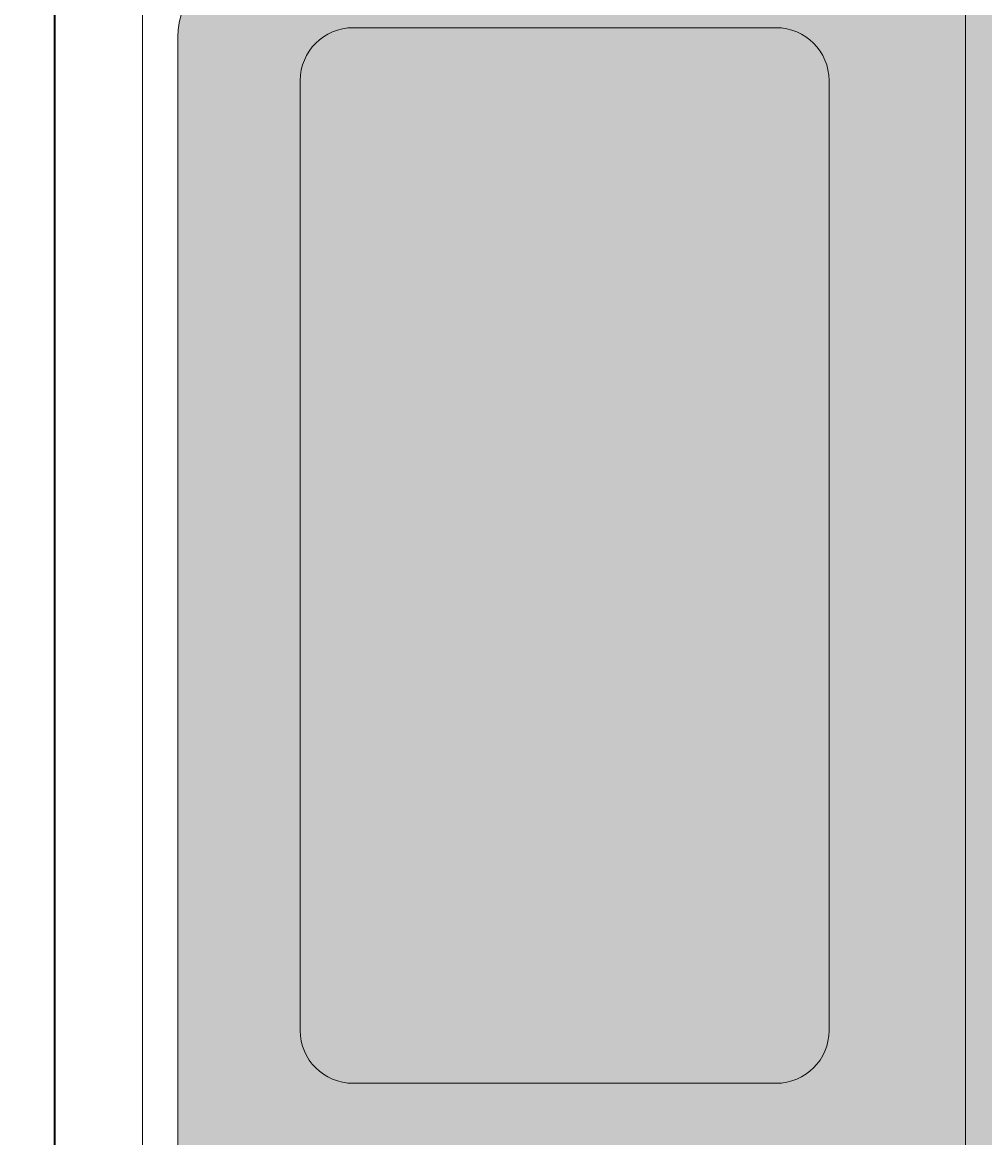
# Model space of a CAD drawing. Units: millimetres. Extents: x 27017497 to 27018854, y 7058029 to 7059154.
# Tile 83 of 91: x 27018319 to 27018341, y 7058530 to 7058555. Entities that reach past the tile are written whole.
import ezdxf

# ---------------------------------------------------------------- set-up
doc = ezdxf.new("R2010")
doc.units = ezdxf.units.MM
for name, color, linetype, lineweight in [('A-ANNO-DIMS', 2, 'Continuous', 18), ('A-FURN', 8, 'Continuous', 18), ('A-WALL', 7, 'Continuous', 35)]:
    doc.layers.add(name, color=color, linetype=linetype, lineweight=lineweight)
doc.layers.add('A-FURN-PATT', color=177, linetype='Continuous', lineweight=13, true_color=0x293189)
doc.styles.get("Standard").update_dxf_attribs({"font": 'arial.ttf'})
doc.dimstyles.get("Standard").update_dxf_attribs({"dimtxt": 0.18, "dimasz": 0.18, "dimexe": 0.18, "dimexo": 0.0625, "dimgap": 0.09, "dimtad": 0, "dimtih": 1, "dimtoh": 1, "dimdec": 4, "dimzin": 0, "dimdsep": 46, "dimtxsty": 'Standard', "dimcen": 0.09, "dimadec": 0, "dimazin": 0, "dimtfac": 1, "dimtdec": 4, "dimtofl": 0, "dimtmove": 0, "dimatfit": 3, "dimfxl": 1, "dimtolj": 1, "dimtzin": 0, "dimarcsym": 0})

# ---------------------------------------------------------------- blocks, each defined once
blk = doc.blocks.new('CAMMAT')
for p, q in [((1.27313, 0), (-1.27313, 0)), ((1.27313, -0.05), (-1.27313, -0.05)), ((0.61, -0.07), (-0.61, -0.07)), ((-0.04645, -0.1395), (-0.58524, -0.1395)), ((-0.61524, -0.1695), (-0.61524, -0.4095)), ((-0.01645, -0.1695), (-0.01645, -0.4095)), ((-0.04645, -0.4395), (-0.58524, -0.4395)), ((-0.6904, -0.51693), (0.68256, -0.51693))]:
    blk.add_line(p, q)
for centre, radius, start, end in [((-0.61, -0.11), 0.04, 90, 180), ((-0.58524, -0.1695), 0.03, 90, 180), ((-0.04645, -0.1695), 0.03, 360, 90), ((-0.58524, -0.4095), 0.03, 180, 270), ((-0.04645, -0.4095), 0.03, 270, 360)]:
    blk.add_arc(centre, radius, start, end)
blk = doc.blocks.new('*D48')
at = {"layer": 'A-ANNO-DIMS', "color": 0, "lineweight": -2, "transparency": 16777216}
for p, q in [((27018463.498, 7058622.912), (27017497.536, 7058622.912)), ((27017497.716, 7058622.732), (27017497.716, 7058357.753)), ((27017497.716, 7058092.41), (27017497.716, 7058357.389)), ((27018555.129, 7058092.23), (27017497.536, 7058092.23))]:
    blk.add_line(p, q, dxfattribs=at)
at = {"layer": 'A-ANNO-DIMS', "color": 0, "transparency": 16777216}
for points in [[(27017497.686, 7058622.732), (27017497.746, 7058622.732), (27017497.716, 7058622.912)], [(27017497.686, 7058092.41), (27017497.746, 7058092.41), (27017497.716, 7058092.23)]]:
    blk.add_solid(points, dxfattribs=at)
at = {"layer": 'Defpoints', "color": 0, "transparency": 16777216}
for p in [(27018463.561, 7058622.912), (27017497.716, 7058092.23), (27018555.192, 7058092.23)]:
    blk.add_point(p, dxfattribs=at)
at = {"layer": 'A-ANNO-DIMS', "color": 0, "transparency": 16777216, "insert": (27017497.716, 7058357.571), "char_height": 0.18, "attachment_point": 5}
blk.add_mtext('\\A1;530.7', dxfattribs=at)
blk = doc.blocks.new('*D50')
at = {"layer": 'A-ANNO-DIMS', "color": 0, "lineweight": -2, "transparency": 16777216}
for p, q in [((27018223.668, 7058580.912), (27018854.236, 7058580.912)), ((27018854.056, 7058580.732), (27018854.056, 7058511.344)), ((27018854.056, 7058441.592), (27018854.056, 7058510.98)), ((27018223.668, 7058441.412), (27018854.236, 7058441.412))]:
    blk.add_line(p, q, dxfattribs=at)
at = {"layer": 'A-ANNO-DIMS', "color": 0, "transparency": 16777216}
for points in [[(27018854.026, 7058580.732), (27018854.086, 7058580.732), (27018854.056, 7058580.912)], [(27018854.026, 7058441.592), (27018854.086, 7058441.592), (27018854.056, 7058441.412)]]:
    blk.add_solid(points, dxfattribs=at)
at = {"layer": 'Defpoints', "color": 0, "transparency": 16777216}
for p in [(27018223.606, 7058580.912), (27018223.606, 7058441.412), (27018854.056, 7058441.412)]:
    blk.add_point(p, dxfattribs=at)
at = {"layer": 'A-ANNO-DIMS', "color": 0, "transparency": 16777216, "insert": (27018854.056, 7058511.162), "char_height": 0.18, "attachment_point": 5}
blk.add_mtext('\\A1;139.5', dxfattribs=at)

msp = doc.modelspace()

# ---------------------------------------------------------------- hatches: boundary and pattern name
at = {"layer": 'A-FURN-PATT'}
h = msp.add_hatch(color=256, dxfattribs=at)
h.dxf.hatch_style = 1
h.paths.add_polyline_path([(27018398.067, 7058554.497, 0.414214), (27018396.474, 7058556.09), (27018352.018, 7058556.09), (27018352.202, 7058552.834), (27018352.581, 7058547.929), (27018353.082, 7058544.346), (27018353.818, 7058541.828), (27018354.899, 7058540.115), (27018356.437, 7058538.948), (27018358.543, 7058538.068), (27018361.329, 7058537.215), (27018358.524, 7058536.613), (27018356.284, 7058536.07), (27018354.381, 7058535.48), (27018352.588, 7058534.736), (27018350.68, 7058533.729), (27018348.431, 7058532.354), (27018345.612, 7058530.503), (27018341.998, 7058528.068), (27018345.612, 7058525.633), (27018348.431, 7058523.782), (27018350.68, 7058522.407), (27018352.588, 7058521.4), (27018354.381, 7058520.656), (27018356.284, 7058520.066), (27018358.524, 7058519.523), (27018361.329, 7058518.92), (27018358.543, 7058518.068), (27018356.437, 7058517.188), (27018354.899, 7058516.021), (27018353.818, 7058514.308), (27018353.082, 7058511.79), (27018352.581, 7058508.207), (27018352.28, 7058504.311), (27018396.474, 7058504.311, 0.414214), (27018398.067, 7058505.904)])
h.paths.add_polyline_path([(27018356.437, 7058538.948), (27018354.899, 7058540.115), (27018353.818, 7058541.828), (27018353.082, 7058544.346), (27018352.581, 7058547.929), (27018352.202, 7058552.834), (27018351.835, 7058559.322), (27018341.998, 7058528.068), (27018345.612, 7058530.503), (27018348.431, 7058532.354), (27018350.68, 7058533.729), (27018352.588, 7058534.736), (27018354.381, 7058535.48), (27018356.284, 7058536.07), (27018358.524, 7058536.613), (27018361.329, 7058537.215), (27018358.543, 7058538.068)])
h.paths.add_polyline_path([(27018358.543, 7058518.068), (27018361.329, 7058518.92), (27018358.524, 7058519.523), (27018356.284, 7058520.066), (27018354.381, 7058520.656), (27018352.588, 7058521.4), (27018350.68, 7058522.407), (27018348.431, 7058523.782), (27018345.612, 7058525.633), (27018341.998, 7058528.068), (27018351.835, 7058496.813), (27018352.202, 7058503.301), (27018352.581, 7058508.207), (27018353.082, 7058511.79), (27018353.818, 7058514.308), (27018354.899, 7058516.021), (27018356.437, 7058517.188)])
h.paths.add_polyline_path([(27018351.324, 7058557.699), (27018340.191, 7058557.699), (27018340.191, 7058503.014), (27018349.884, 7058503.014), (27018341.998, 7058528.068)])
h.paths.add_polyline_path([(27018340.191, 7058556.09), (27018323.983, 7058556.09, 0.414214), (27018322.39, 7058554.497), (27018322.39, 7058505.904, 0.414214), (27018323.983, 7058504.311), (27018340.191, 7058504.311)])
h.paths.add_polyline_path([(27018337.107, 7058532.051, -0.414214), (27018335.912, 7058530.856), (27018326.353, 7058530.856, -0.414214), (27018325.158, 7058532.051), (27018325.158, 7058553.51, -0.414214), (27018326.353, 7058554.705), (27018335.912, 7058554.705, -0.414214), (27018337.107, 7058553.51)], flags=0)
h.paths.add_polyline_path([(27018337.107, 7058527.914), (27018337.107, 7058506.454, -0.414214), (27018335.912, 7058505.259), (27018326.353, 7058505.259, -0.414214), (27018325.158, 7058506.454), (27018325.158, 7058527.914, -0.414214), (27018326.353, 7058529.109), (27018335.912, 7058529.109, -0.414214)], flags=0)
h.paths.add_polyline_path([(27018338.322, 7058577.2), (27018322.39, 7058577.2), (27018322.39, 7058557.285), (27018338.322, 7058557.285)])
h.paths.add_polyline_path([(27018323.748, 7058567.284, -1), (27018335.697, 7058567.284, -1)], flags=16)
h.paths.add_polyline_path([(27018326.023, 7058567.284, -1), (27018333.423, 7058567.284, -1)], flags=0)
h.paths.add_polyline_path([(27018338.322, 7058503.116), (27018322.39, 7058503.116), (27018322.39, 7058483.201), (27018338.322, 7058483.201)])
h.paths.add_polyline_path([(27018335.697, 7058493.391, -1), (27018323.748, 7058493.391, -1)], flags=16)
h.paths.add_polyline_path([(27018333.423, 7058493.391, -1), (27018326.023, 7058493.391, -1)], flags=0)
h.paths.add_polyline_path([(27018337.107, 7058527.914, 0.414214), (27018335.912, 7058529.109), (27018326.353, 7058529.109, 0.414214), (27018325.158, 7058527.914), (27018325.158, 7058506.454, 0.414214), (27018326.353, 7058505.259), (27018335.912, 7058505.259, 0.414214), (27018337.107, 7058506.454)], flags=16)
h.paths.add_polyline_path([(27018337.107, 7058553.51, 0.414214), (27018335.912, 7058554.705), (27018326.353, 7058554.705, 0.414214), (27018325.158, 7058553.51), (27018325.158, 7058532.051, 0.414214), (27018326.353, 7058530.856), (27018335.912, 7058530.856, 0.414214), (27018337.107, 7058532.051)], flags=16)
h = msp.add_hatch(color=256, dxfattribs=at)
h.dxf.hatch_style = 1
h.paths.add_polyline_path([(27018337.107, 7058553.51, 0.414214), (27018335.912, 7058554.705), (27018326.353, 7058554.705, 0.414214), (27018325.158, 7058553.51), (27018325.158, 7058532.051, 0.414214), (27018326.353, 7058530.856), (27018335.912, 7058530.856, 0.414214), (27018337.107, 7058532.051)])
h.paths.add_polyline_path([(27018337.107, 7058527.914, 0.414214), (27018335.912, 7058529.109), (27018326.353, 7058529.109, 0.414214), (27018325.158, 7058527.914), (27018325.158, 7058506.454, 0.414214), (27018326.353, 7058505.259), (27018335.912, 7058505.259, 0.414214), (27018337.107, 7058506.454)])

# ---------------------------------------------------------------- linework, layer by layer
at = {"layer": 'A-WALL'}
msp.add_line((27018319.606, 7058580.912), (27018319.606, 7058412.636), dxfattribs=at)

# ---------------------------------------------------------------- block references
at = {"layer": 'A-FURN', "xscale": -39.82996475819422, "yscale": 39.82996475819422, "zscale": 39.82996475819422, "rotation": 90}
msp.add_blockref('CAMMAT', (27018319.602, 7058530.2), dxfattribs=at)

# ---------------------------------------------------------------- dimensions: what is measured, and where the dimension line sits
at = {"layer": 'A-ANNO-DIMS'}
for base, p1, p2, picture, middle in [((27017497.716, 7058092.23), (27018463.561, 7058622.912), (27018555.192, 7058092.23), '*D48', (27017497.716, 7058357.571)), ((27018854.056, 7058441.412), (27018223.606, 7058580.912), (27018223.606, 7058441.412), '*D50', (27018854.056, 7058511.162))]:
    dim = msp.add_linear_dim(base=base, p1=p1, p2=p2, angle=90, dimstyle='Standard', override={"dimdec": 1, "dimlfac": 1, "dimrnd": 0, "dimzin": 0, "dimdsep": 46, "dimlunit": 2}, dxfattribs=at)
    dim.commit()
    dim.dimension.update_dxf_attribs({"geometry": picture, "text_midpoint": middle})

doc.saveas('drawing.dxf')
